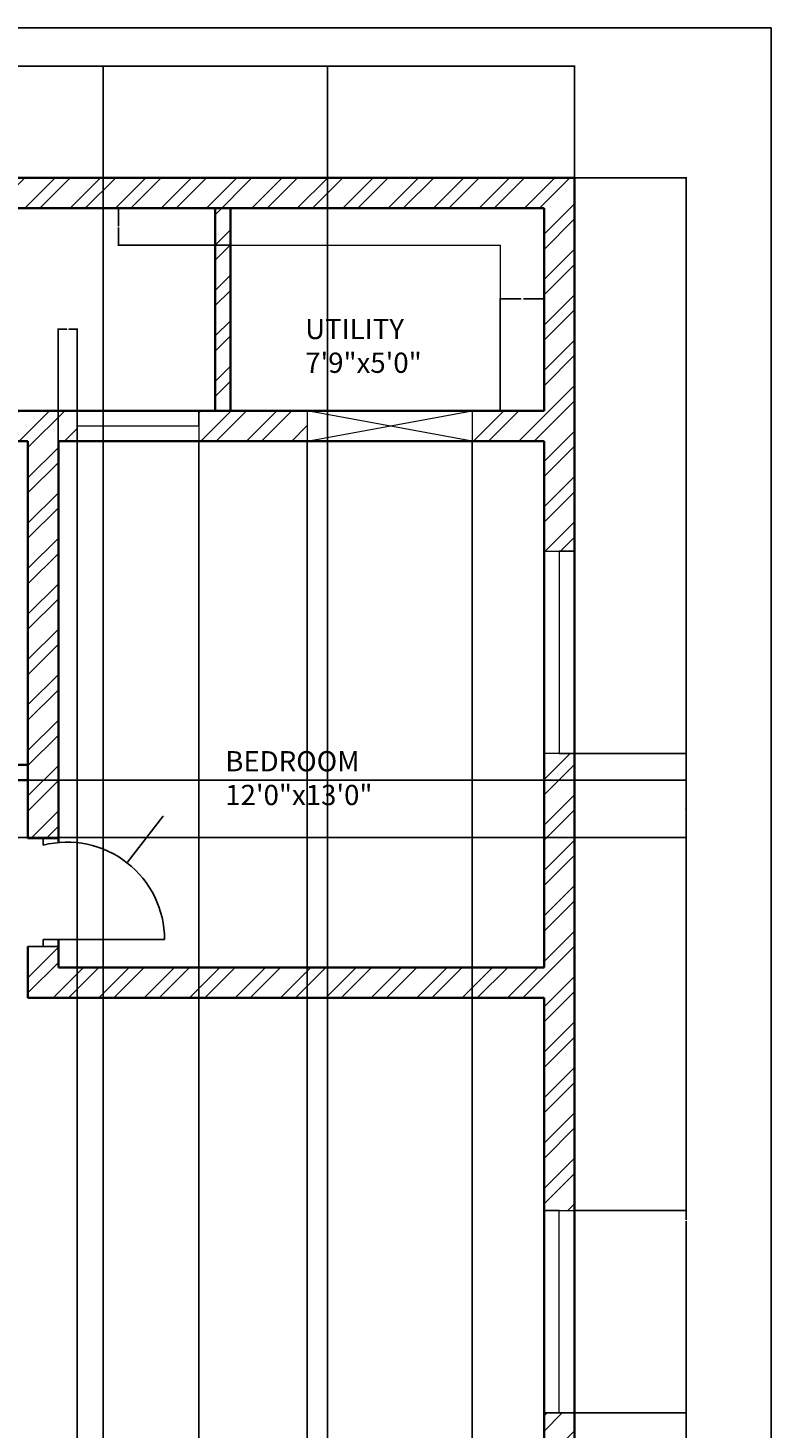
# Model space of a CAD drawing. Units: inches. Extents: x 1595 to 2135, y 460 to 2061.
# Tile 5 of 5: x 1914 to 2135, y 1646 to 2061. Entities that reach past the tile are written whole.
import ezdxf

# ---------------------------------------------------------------- set-up
doc = ezdxf.new("R2010")
doc.units = ezdxf.units.IN
for name, color, linetype, lineweight in [('A-ANNO-DIMS', 2, 'Continuous', 18), ('A-ANNO-TTLB', 7, 'Continuous', 25), ('A-AREA-IDEN', 7, 'Continuous', 18), ('A-DOOR', 3, 'Continuous', 25), ('A-FLOR-FIXT', 9, 'Continuous', 18), ('A-GLAZ', 4, 'Continuous', 18), ('A-WALL', 7, 'Continuous', 35)]:
    doc.layers.add(name, color=color, linetype=linetype, lineweight=lineweight)
doc.layers.add('A-WALL-PATT', color=143, linetype='Continuous', lineweight=13, true_color=0x7aafdf)
doc.styles.get("Standard").update_dxf_attribs({"font": 'arial.ttf'})
doc.dimstyles.get("Standard").update_dxf_attribs({"dimtxt": 0.18, "dimasz": 0.18, "dimexe": 0.18, "dimexo": 0.0625, "dimgap": 0.09, "dimtad": 0, "dimtih": 1, "dimtoh": 1, "dimdec": 4, "dimzin": 0, "dimdsep": 46, "dimtxsty": 'Standard', "dimcen": 0.09, "dimadec": 0, "dimazin": 0, "dimtfac": 1, "dimtdec": 4, "dimtofl": 0, "dimtmove": 0, "dimatfit": 3, "dimfxl": 1, "dimtolj": 1, "dimtzin": 0, "dimarcsym": 0})

# ---------------------------------------------------------------- blocks, each defined once
blk = doc.blocks.new('*D7')
at = {"layer": 'A-ANNO-DIMS', "color": 0, "lineweight": -2, "transparency": 16777216}
for p, q in [((1923.31, 1938.7), (1923.31, 1971.97)), ((1923.49, 1971.79), (1925.8, 1971.79)), ((1928.75, 1971.79), (1926.45, 1971.79)), ((1928.93, 1938.7), (1928.93, 1971.97))]:
    blk.add_line(p, q, dxfattribs=at)
at = {"layer": 'A-ANNO-DIMS', "color": 0, "transparency": 16777216}
for points in [[(1923.49, 1971.82), (1923.49, 1971.76), (1923.31, 1971.79)], [(1928.75, 1971.82), (1928.75, 1971.76), (1928.93, 1971.79)]]:
    blk.add_solid(points, dxfattribs=at)
at = {"layer": 'Defpoints', "color": 0, "transparency": 16777216}
for p in [(1928.93, 1971.79), (1923.31, 1938.64), (1928.93, 1938.64)]:
    blk.add_point(p, dxfattribs=at)
at = {"layer": 'A-ANNO-DIMS', "color": 0, "transparency": 16777216, "insert": (1926.12, 1971.79), "char_height": 0.18, "attachment_point": 5}
blk.add_mtext('\\A1;5.62', dxfattribs=at)
blk = doc.blocks.new('*D15')
at = {"layer": 'A-ANNO-DIMS', "color": 0, "lineweight": -2, "transparency": 16777216}
for p, q in [((2076.38, 1650.64), (2109.64, 1650.64)), ((2109.46, 1650.46), (2109.46, 1577.6)), ((2109.46, 1504.38), (2109.46, 1577.24)), ((2076.38, 1504.2), (2109.64, 1504.2))]:
    blk.add_line(p, q, dxfattribs=at)
at = {"layer": 'A-ANNO-DIMS', "color": 0, "transparency": 16777216}
for points in [[(2109.43, 1650.46), (2109.49, 1650.46), (2109.46, 1650.64)], [(2109.43, 1504.38), (2109.49, 1504.38), (2109.46, 1504.2)]]:
    blk.add_solid(points, dxfattribs=at)
at = {"layer": 'Defpoints', "color": 0, "transparency": 16777216}
for p in [(2076.31, 1650.64), (2109.46, 1650.64), (2076.31, 1504.2)]:
    blk.add_point(p, dxfattribs=at)
at = {"layer": 'A-ANNO-DIMS', "color": 0, "transparency": 16777216, "insert": (2109.46, 1577.42), "char_height": 0.18, "attachment_point": 5}
blk.add_mtext('\\A1;146.44', dxfattribs=at)
blk = doc.blocks.new('*D16')
at = {"layer": 'A-ANNO-DIMS', "color": 0, "lineweight": -2, "transparency": 16777216}
for p, q in [((2076.38, 1846.04), (2109.64, 1846.04)), ((2109.46, 1845.86), (2109.46, 1778.52)), ((2109.46, 1710.82), (2109.46, 1778.16)), ((2076.38, 1710.64), (2109.64, 1710.64))]:
    blk.add_line(p, q, dxfattribs=at)
at = {"layer": 'A-ANNO-DIMS', "color": 0, "transparency": 16777216}
for points in [[(2109.43, 1845.86), (2109.49, 1845.86), (2109.46, 1846.04)], [(2109.43, 1710.82), (2109.49, 1710.82), (2109.46, 1710.64)]]:
    blk.add_solid(points, dxfattribs=at)
at = {"layer": 'Defpoints', "color": 0, "transparency": 16777216}
for p in [(2076.31, 1846.04), (2109.46, 1846.04), (2076.31, 1710.64)]:
    blk.add_point(p, dxfattribs=at)
at = {"layer": 'A-ANNO-DIMS', "color": 0, "transparency": 16777216, "insert": (2109.46, 1778.34), "char_height": 0.18, "attachment_point": 5}
blk.add_mtext('\\A1;135.4', dxfattribs=at)
blk = doc.blocks.new('*D21')
at = {"layer": 'A-ANNO-DIMS', "color": 0, "lineweight": -2, "transparency": 16777216}
for p, q in [((1936.61, 1577.2), (1936.61, 2049.97)), ((1936.79, 2049.79), (1969.47, 2049.79)), ((2002.95, 2049.79), (1970.26, 2049.79)), ((2003.13, 1577.2), (2003.13, 2049.97))]:
    blk.add_line(p, q, dxfattribs=at)
at = {"layer": 'A-ANNO-DIMS', "color": 0, "transparency": 16777216}
for points in [[(1936.79, 2049.82), (1936.79, 2049.76), (1936.61, 2049.79)], [(2002.95, 2049.82), (2002.95, 2049.76), (2003.13, 2049.79)]]:
    blk.add_solid(points, dxfattribs=at)
at = {"layer": 'Defpoints', "color": 0, "transparency": 16777216}
for p in [(2003.13, 2049.79), (1936.61, 1577.14), (2003.13, 1577.14)]:
    blk.add_point(p, dxfattribs=at)
at = {"layer": 'A-ANNO-DIMS', "color": 0, "transparency": 16777216, "insert": (1969.87, 2049.79), "char_height": 0.18, "attachment_point": 5}
blk.add_mtext('\\A1;66.52', dxfattribs=at)
blk = doc.blocks.new('*D27')
at = {"layer": 'A-ANNO-DIMS', "color": 0, "lineweight": -2, "transparency": 16777216}
for p, q in [((1997.11, 1938.58), (1997.11, 1365.31)), ((2046.03, 1938.58), (2046.03, 1365.31)), ((1997.29, 1365.49), (2021.18, 1365.49)), ((2045.85, 1365.49), (2021.97, 1365.49))]:
    blk.add_line(p, q, dxfattribs=at)
at = {"layer": 'A-ANNO-DIMS', "color": 0, "transparency": 16777216}
for points in [[(1997.29, 1365.52), (1997.29, 1365.46), (1997.11, 1365.49)], [(2045.85, 1365.52), (2045.85, 1365.46), (2046.03, 1365.49)]]:
    blk.add_solid(points, dxfattribs=at)
at = {"layer": 'Defpoints', "color": 0, "transparency": 16777216}
for p in [(1997.11, 1938.64), (2046.03, 1938.64), (2046.03, 1365.49)]:
    blk.add_point(p, dxfattribs=at)
at = {"layer": 'A-ANNO-DIMS', "color": 0, "transparency": 16777216, "insert": (2021.57, 1365.49), "char_height": 0.18, "attachment_point": 5}
blk.add_mtext('\\A1;48.92', dxfattribs=at)
blk = doc.blocks.new('*D28')
at = {"layer": 'A-ANNO-DIMS', "color": 0, "lineweight": -2, "transparency": 16777216}
for p, q in [((1928.93, 1938.58), (1928.93, 1365.31)), ((1964.93, 1938.58), (1964.93, 1365.31)), ((1929.11, 1365.49), (1946.71, 1365.49)), ((1964.75, 1365.49), (1947.15, 1365.49))]:
    blk.add_line(p, q, dxfattribs=at)
at = {"layer": 'A-ANNO-DIMS', "color": 0, "transparency": 16777216}
for points in [[(1929.11, 1365.52), (1929.11, 1365.46), (1928.93, 1365.49)], [(1964.75, 1365.52), (1964.75, 1365.46), (1964.93, 1365.49)]]:
    blk.add_solid(points, dxfattribs=at)
at = {"layer": 'Defpoints', "color": 0, "transparency": 16777216}
for p in [(1928.93, 1938.64), (1964.93, 1938.64), (1964.93, 1365.49)]:
    blk.add_point(p, dxfattribs=at)
at = {"layer": 'A-ANNO-DIMS', "color": 0, "transparency": 16777216, "insert": (1946.93, 1365.49), "char_height": 0.18, "attachment_point": 5}
blk.add_mtext('\\A1;36', dxfattribs=at)
blk = doc.blocks.new('*D29')
at = {"layer": 'A-ANNO-DIMS', "color": 0, "lineweight": -2, "transparency": 16777216}
for p, q in [((1964.93, 1938.58), (1964.93, 1365.31)), ((1997.11, 1938.58), (1997.11, 1365.31)), ((1965.11, 1365.49), (1980.63, 1365.49)), ((1996.93, 1365.49), (1981.42, 1365.49))]:
    blk.add_line(p, q, dxfattribs=at)
at = {"layer": 'A-ANNO-DIMS', "color": 0, "transparency": 16777216}
for points in [[(1965.11, 1365.52), (1965.11, 1365.46), (1964.93, 1365.49)], [(1996.93, 1365.52), (1996.93, 1365.46), (1997.11, 1365.49)]]:
    blk.add_solid(points, dxfattribs=at)
at = {"layer": 'Defpoints', "color": 0, "transparency": 16777216}
for p in [(1964.93, 1938.64), (1997.11, 1938.64), (1997.11, 1365.49)]:
    blk.add_point(p, dxfattribs=at)
at = {"layer": 'A-ANNO-DIMS', "color": 0, "transparency": 16777216, "insert": (1981.02, 1365.49), "char_height": 0.18, "attachment_point": 5}
blk.add_mtext('\\A1;32.18', dxfattribs=at)
blk = doc.blocks.new('*D31')
at = {"layer": 'A-ANNO-DIMS', "color": 0, "lineweight": -2, "transparency": 16777216}
for p, q in [((1836.38, 1838.14), (2109.64, 1838.14)), ((2109.46, 1837.96), (2109.46, 1829.81)), ((2109.46, 1821.29), (2109.46, 1829.44)), ((1836.38, 1821.11), (2109.64, 1821.11))]:
    blk.add_line(p, q, dxfattribs=at)
at = {"layer": 'A-ANNO-DIMS', "color": 0, "transparency": 16777216}
for points in [[(2109.43, 1837.96), (2109.49, 1837.96), (2109.46, 1838.14)], [(2109.43, 1821.29), (2109.49, 1821.29), (2109.46, 1821.11)]]:
    blk.add_solid(points, dxfattribs=at)
at = {"layer": 'Defpoints', "color": 0, "transparency": 16777216}
for p in [(1836.31, 1838.14), (1836.31, 1821.11), (2109.46, 1821.11)]:
    blk.add_point(p, dxfattribs=at)
at = {"layer": 'A-ANNO-DIMS', "color": 0, "transparency": 16777216, "insert": (2109.46, 1829.63), "char_height": 0.18, "attachment_point": 5}
blk.add_mtext('\\A1;17.034', dxfattribs=at)
blk = doc.blocks.new('*D45')
at = {"layer": 'A-ANNO-DIMS', "color": 0, "lineweight": -2, "transparency": 16777216}
for p, q in [((1674.31, 2016.7), (1674.31, 2049.97)), ((1674.49, 2049.79), (1875.02, 2049.79)), ((2076.13, 2049.79), (1875.6, 2049.79)), ((2076.31, 2016.7), (2076.31, 2049.97))]:
    blk.add_line(p, q, dxfattribs=at)
at = {"layer": 'A-ANNO-DIMS', "color": 0, "transparency": 16777216}
for points in [[(1674.49, 2049.82), (1674.49, 2049.76), (1674.31, 2049.79)], [(2076.13, 2049.82), (2076.13, 2049.76), (2076.31, 2049.79)]]:
    blk.add_solid(points, dxfattribs=at)
at = {"layer": 'Defpoints', "color": 0, "transparency": 16777216}
for p in [(2076.31, 2049.79), (1674.31, 2016.64), (2076.31, 2016.64)]:
    blk.add_point(p, dxfattribs=at)
at = {"layer": 'A-ANNO-DIMS', "color": 0, "transparency": 16777216, "insert": (1875.31, 2049.79), "char_height": 0.18, "attachment_point": 5}
blk.add_mtext('\\A1;402', dxfattribs=at)
blk = doc.blocks.new('*D46')
at = {"layer": 'A-ANNO-DIMS', "color": 0, "lineweight": -2, "transparency": 16777216}
for p, q in [((2076.38, 2016.64), (2109.64, 2016.64)), ((2109.46, 2016.46), (2109.46, 1707.82)), ((2109.46, 1398.82), (2109.46, 1707.46)), ((2076.38, 1398.64), (2109.64, 1398.64))]:
    blk.add_line(p, q, dxfattribs=at)
at = {"layer": 'A-ANNO-DIMS', "color": 0, "transparency": 16777216}
for points in [[(2109.43, 2016.46), (2109.49, 2016.46), (2109.46, 2016.64)], [(2109.43, 1398.82), (2109.49, 1398.82), (2109.46, 1398.64)]]:
    blk.add_solid(points, dxfattribs=at)
at = {"layer": 'Defpoints', "color": 0, "transparency": 16777216}
for p in [(2076.31, 2016.64), (2109.46, 2016.64), (2076.31, 1398.64)]:
    blk.add_point(p, dxfattribs=at)
at = {"layer": 'A-ANNO-DIMS', "color": 0, "transparency": 16777216, "insert": (2109.46, 1707.64), "char_height": 0.18, "attachment_point": 5}
blk.add_mtext('\\A1;618', dxfattribs=at)
blk = doc.blocks.new('*D51')
at = {"layer": 'A-ANNO-DIMS', "color": 0, "lineweight": -2, "transparency": 16777216}
for p, q in [((2054.32, 1947.7), (2054.32, 1980.97)), ((2054.5, 1980.79), (2060.43, 1980.79)), ((2067.13, 1980.79), (2061.2, 1980.79)), ((2067.31, 1947.7), (2067.31, 1980.97))]:
    blk.add_line(p, q, dxfattribs=at)
at = {"layer": 'A-ANNO-DIMS', "color": 0, "transparency": 16777216}
for points in [[(2054.5, 1980.82), (2054.5, 1980.76), (2054.32, 1980.79)], [(2067.13, 1980.82), (2067.13, 1980.76), (2067.31, 1980.79)]]:
    blk.add_solid(points, dxfattribs=at)
at = {"layer": 'Defpoints', "color": 0, "transparency": 16777216}
for p in [(2067.31, 1980.79), (2054.32, 1947.64), (2067.31, 1947.64)]:
    blk.add_point(p, dxfattribs=at)
at = {"layer": 'A-ANNO-DIMS', "color": 0, "transparency": 16777216, "insert": (2060.82, 1980.79), "char_height": 0.18, "attachment_point": 5}
blk.add_mtext('\\A1;12.99', dxfattribs=at)
blk = doc.blocks.new('*D52')
at = {"layer": 'A-ANNO-DIMS', "color": 0, "lineweight": -2, "transparency": 16777216}
for p, q in [((1974.25, 2007.64), (1940.98, 2007.64)), ((1941.16, 2007.46), (1941.16, 2002.33)), ((1941.16, 1996.84), (1941.16, 2001.97)), ((1974.25, 1996.66), (1940.98, 1996.66))]:
    blk.add_line(p, q, dxfattribs=at)
at = {"layer": 'A-ANNO-DIMS', "color": 0, "transparency": 16777216}
for points in [[(1941.13, 2007.46), (1941.19, 2007.46), (1941.16, 2007.64)], [(1941.13, 1996.84), (1941.19, 1996.84), (1941.16, 1996.66)]]:
    blk.add_solid(points, dxfattribs=at)
at = {"layer": 'Defpoints', "color": 0, "transparency": 16777216}
for p in [(1941.16, 2007.64), (1974.31, 2007.64), (1974.31, 1996.66)]:
    blk.add_point(p, dxfattribs=at)
at = {"layer": 'A-ANNO-DIMS', "color": 0, "transparency": 16777216, "insert": (1941.16, 2002.15), "char_height": 0.18, "attachment_point": 5}
blk.add_mtext('\\A1;10.98', dxfattribs=at)
blk = doc.blocks.new('*D57')
at = {"layer": 'A-ANNO-DIMS', "color": 0, "lineweight": -2, "transparency": 16777216}
for p, q in [((1954.31, 1827.37), (1943.77, 1813.83)), ((1954.49, 1827.37), (1954.31, 1827.37)), ((1925.83, 1790.88), (1926.01, 1790.88)), ((1925.92, 1790.79), (1925.92, 1790.97))]:
    blk.add_line(p, q, dxfattribs=at)
at = {"layer": 'A-ANNO-DIMS', "color": 0, "transparency": 16777216}
blk.add_solid([(1943.75, 1813.85), (1943.8, 1813.81), (1943.66, 1813.69)], dxfattribs=at)
at = {"layer": 'Defpoints', "color": 0, "transparency": 16777216}
for p in [(1943.66, 1813.69), (1925.92, 1790.88)]:
    blk.add_point(p, dxfattribs=at)
at = {"layer": 'A-ANNO-DIMS', "color": 0, "transparency": 16777216, "insert": (1955.04, 1827.37), "char_height": 0.18, "attachment_point": 5}
blk.add_mtext('\\A1;R28.896', dxfattribs=at)

msp = doc.modelspace()

# ---------------------------------------------------------------- hatches: boundary and pattern name
at = {"layer": 'A-WALL-PATT'}
h = msp.add_hatch(dxfattribs=at)
h.set_pattern_fill('ANSI32', color=256)
h.paths.add_polyline_path([(2076.313, 2016.6421), (1674.313, 2016.6421), (1674.313, 1905.0731), (1683.313, 1905.0731), (1683.313, 1938.6421), (1705.9756, 1938.6421), (1705.9756, 1947.6421), (1683.313, 1947.6421), (1683.313, 2007.6421), (2067.313, 2007.6421), (2067.313, 1947.6421), (2046.0304, 1947.6421), (2046.0304, 1938.6421), (2067.313, 1938.6421), (2067.313, 1906.0373), (2076.313, 1906.0373), (2076.313, 1947.6421)])
h.paths.add_polyline_path([(1786.653, 1947.6421), (1748.8699, 1947.6421), (1748.8699, 1938.6421), (1786.653, 1938.6421), (1786.653, 1943.1421)], flags=17)
h.paths.add_polyline_path([(1843.367, 1943.1421), (1843.367, 1947.6421), (1822.653, 1947.6421), (1822.653, 1938.6421), (1827.313, 1938.6421), (1827.313, 1821.1082), (1836.313, 1821.1082), (1836.313, 1938.6421), (1843.367, 1938.6421)])
h.paths.add_polyline_path([(1928.933, 1943.1421), (1928.933, 1947.6421), (1875.313, 1947.6421), (1875.313, 1938.6421), (1914.313, 1938.6421), (1914.313, 1820.8892), (1923.313, 1820.8892), (1923.313, 1938.6421), (1928.933, 1938.6421)])
h.paths.add_polyline_path([(1997.1133, 1947.6421), (1964.933, 1947.6421), (1964.933, 1938.6421), (1997.1133, 1938.6421)], flags=17)
h.paths.add_polyline_path([(1974.313, 2007.6421), (1969.813, 2007.6421), (1969.813, 1947.6421), (1974.313, 1947.6421)], flags=17)
h.paths.add_polyline_path([(1780.813, 2007.6421), (1776.313, 2007.6421), (1776.313, 1947.6421), (1780.813, 1947.6421)], flags=17)
h.paths.add_polyline_path([(1683.313, 1845.0731), (1674.313, 1845.0731), (1674.313, 1734.209), (1683.313, 1734.209), (1683.313, 1773.6421), (1795.813, 1773.6421), (1836.313, 1773.6421), (1836.313, 1788.3627), (1831.813, 1788.3627), (1827.313, 1788.3627), (1827.313, 1782.6421), (1683.313, 1782.6421)])
h.paths.add_polyline_path([(2076.313, 1846.0373), (2067.313, 1846.0373), (2067.313, 1782.6421), (1923.313, 1782.6421), (1923.313, 1788.8802), (1918.813, 1788.8802), (1914.313, 1788.8802), (1914.313, 1773.6421), (2067.313, 1773.6421), (2067.313, 1710.6421), (2076.313, 1710.6421)])
h.paths.add_polyline_path([(1844.0531, 1859.9747), (1909.4596, 1859.9747), (1909.4596, 1882.3635), (1844.0531, 1882.3635)], flags=9)
h.paths.add_polyline_path([(1721.6058, 1827.3507), (1768.2143, 1827.3507), (1768.2143, 1849.7395), (1721.6058, 1849.7395)], flags=9)
h.paths.add_polyline_path([(1786.8661, 1359.2872), (1978.2276, 1359.2872), (1978.2276, 1384.0157), (1786.8661, 1384.0157)], flags=9)
h.paths.add_polyline_path([(1795.7228, 1412.0413), (1871.5904, 1412.0413), (1871.5904, 1424.4055), (1795.7228, 1424.4055)], flags=9)
h.paths.add_polyline_path([(1954.3634, 1526.3976), (2013.549, 1526.3976), (2013.549, 1548.7864), (1954.3634, 1548.7864)], flags=9)
h.paths.add_polyline_path([(1871.0596, 1490.4707), (1913.1292, 1490.4707), (1913.1292, 1512.8595), (1871.0596, 1512.8595)], flags=9)
h.paths.add_polyline_path([(1810.9452, 1510.8402), (1845.9343, 1510.8402), (1845.9343, 1533.229), (1810.9452, 1533.229)], flags=9)
h.paths.add_polyline_path([(1720.9117, 1692.9695), (1767.819, 1692.9695), (1767.819, 1715.3583), (1720.9117, 1715.3583)], flags=9)
h.paths.add_polyline_path([(1853.0254, 1698.4614), (1904.6966, 1698.4614), (1904.6966, 1720.8503), (1853.0254, 1720.8503)], flags=9)
h.paths.add_polyline_path([(1970.399, 1827.3507), (2017.0075, 1827.3507), (2017.0075, 1849.7395), (1970.399, 1849.7395)], flags=9)
h.paths.add_polyline_path([(1994.3418, 1955.5613), (2029.5928, 1955.5613), (2029.5928, 1977.9501), (1994.3418, 1977.9501)], flags=25)
h.paths.add_polyline_path([(1828.8665, 1964.6116), (1868.5173, 1964.6116), (1868.5173, 1987.0004), (1828.8665, 1987.0004)], flags=25)
h.paths.add_polyline_path([(1698.1483, 1960.8371), (1733.3994, 1960.8371), (1733.3994, 1983.2259), (1698.1483, 1983.2259)], flags=25)
h = msp.add_hatch(dxfattribs=at)
h.set_pattern_fill('ANSI32', color=256)
h.paths.add_polyline_path([(1683.313, 1641.6421), (1791.313, 1641.6421), (1791.313, 1634.7169), (1800.313, 1634.7169), (1800.313, 1650.6421), (1800.313, 1673.3054), (1795.813, 1673.3054), (1795.813, 1650.6421), (1683.313, 1650.6421), (1683.313, 1698.209), (1678.813, 1698.209), (1674.313, 1698.209), (1674.313, 1398.6421), (1688.853, 1398.6421), (1688.853, 1403.1421), (1688.853, 1407.6421), (1683.313, 1407.6421)])
h.paths.add_polyline_path([(1800.313, 1568.1421), (1827.2399, 1568.1421), (1827.2399, 1572.6421), (1827.2399, 1577.1421), (1800.313, 1577.1421), (1800.313, 1604.9472), (1795.813, 1604.9472), (1791.313, 1604.9472), (1791.313, 1437.6421), (1800.313, 1437.6421), (1815.6708, 1437.6421), (1815.6708, 1442.1421), (1815.6708, 1446.6421), (1800.313, 1446.6421)])
h.paths.add_polyline_path([(1877.5816, 1545.4284), (1877.5816, 1548.9761), (1864.813, 1548.9761), (1864.813, 1577.1421), (1852.144, 1577.1421), (1852.144, 1568.1421), (1860.313, 1568.1421), (1860.313, 1446.6421), (1839.6708, 1446.6421), (1839.6708, 1437.6421), (1869.0647, 1437.6421), (1869.0647, 1442.1421), (1869.0647, 1446.6421), (1864.813, 1446.6421), (1864.813, 1539.9761), (1877.5816, 1539.9761), (1877.5816, 1541.8808)])
h.paths.add_polyline_path([(1923.313, 1568.1421), (1936.607, 1568.1421), (1936.607, 1577.1421), (1914.313, 1577.1421), (1914.313, 1548.9761), (1901.5816, 1548.9761), (1901.5816, 1539.9761), (1914.313, 1539.9761), (1914.313, 1446.6421), (1891.5684, 1446.6421), (1891.5684, 1437.6421), (1914.313, 1437.6421), (1923.313, 1437.6421)])
h.paths.add_polyline_path([(2067.313, 1577.1421), (2003.1294, 1577.1421), (2003.1294, 1568.1421), (2067.313, 1568.1421)])
h.paths.add_polyline_path([(2076.313, 1650.6421), (2067.313, 1650.6421), (2067.313, 1504.2035), (2076.313, 1504.2035)])
h.paths.add_polyline_path([(2076.313, 1444.2035), (2071.813, 1444.2035), (2067.313, 1444.2035), (2067.313, 1407.6421), (1923.313, 1407.6421), (1918.813, 1407.6421), (1914.313, 1407.6421), (1737.2767, 1407.6421), (1737.2767, 1398.6421), (2076.313, 1398.6421)])

# ---------------------------------------------------------------- linework, layer by layer
at = {"layer": 'A-ANNO-TTLB'}
msp.add_lwpolyline([(1595.2754, 2061.0707), (2134.6206, 2061.0707), (2134.6206, 1319.9937), (1595.2754, 1319.9937)], close=True, dxfattribs=at)
at = {"layer": 'A-DOOR'}
for p, q in [((1914.313, 1820.8892), (1923.313, 1820.8892)), ((1923.313, 1820.8892), (1918.813, 1820.8892)), ((1918.813, 1820.8892), (1918.813, 1818.8892)), ((1914.313, 1788.8802), (1923.313, 1788.8802)), ((1918.813, 1788.8802), (1918.813, 1790.8802)), ((1918.813, 1790.8802), (1954.813, 1790.8802)), ((1918.813, 1790.8802), (1954.813, 1790.8802)), ((1923.313, 1788.8802), (1918.813, 1788.8802))]:
    msp.add_line(p, q, dxfattribs=at)
msp.add_arc((1925.9171, 1790.8802), 28.8959, 360, 104.232183, dxfattribs=at)
at = {"layer": 'A-FLOR-FIXT'}
for p, q in [((1974.313, 1996.6616), (2054.323, 1996.6616)), ((2054.323, 1996.6616), (2054.323, 1947.6421))]:
    msp.add_line(p, q, dxfattribs=at)
at = {"layer": 'A-GLAZ'}
for p, q in [((1928.933, 1947.6421), (1928.933, 1938.6421)), ((1964.933, 1943.1421), (1964.933, 1947.6421)), ((1964.933, 1947.6421), (1964.933, 1938.6421)), ((1997.1133, 1947.6421), (1997.1133, 1938.6421)), ((2046.0304, 1938.6421), (1997.1133, 1947.6421)), ((1997.1133, 1947.6421), (1997.1133, 1947.6421)), ((1997.1133, 1938.6421), (2046.0304, 1947.6421)), ((2046.0304, 1947.6421), (2046.0304, 1938.6421)), ((1928.933, 1938.6421), (1928.933, 1943.1421)), ((1928.933, 1943.1421), (1964.933, 1943.1421)), ((1997.1133, 1938.6421), (1997.1133, 1938.6421)), ((2046.0304, 1938.6421), (2046.0304, 1938.6421)), ((2067.313, 1906.0373), (2076.313, 1906.0373)), ((2076.313, 1906.0373), (2071.813, 1906.0373)), ((2071.813, 1906.0373), (2071.813, 1846.0373)), ((2076.313, 1846.0373), (2067.313, 1846.0373)), ((2071.813, 1846.0373), (2076.313, 1846.0373)), ((2071.813, 1710.6421), (2067.313, 1710.6421)), ((2067.313, 1710.6421), (2076.313, 1710.6421)), ((2071.813, 1650.6421), (2071.813, 1710.6421)), ((2067.313, 1650.6421), (2076.313, 1650.6421)), ((2076.313, 1650.6421), (2067.313, 1650.6421))]:
    msp.add_line(p, q, dxfattribs=at)
at = {"layer": 'A-WALL'}
for p, q in [((1674.313, 2016.6421), (2076.313, 2016.6421)), ((2076.313, 2016.6421), (2076.313, 1947.6421)), ((1683.313, 2007.6421), (2067.313, 2007.6421)), ((1969.813, 2007.6421), (1969.813, 1947.6421)), ((1974.313, 2007.6421), (1974.313, 1947.6421)), ((2067.313, 2007.6421), (2067.313, 1947.6421)), ((1875.313, 1947.6421), (2067.313, 1947.6421)), ((2076.313, 1947.6421), (2076.313, 1398.6421)), ((1874.0917, 1938.6421), (1914.313, 1938.6421)), ((1914.313, 1938.6421), (1914.313, 1820.8892)), ((1923.313, 1938.6421), (1923.313, 1819.6585)), ((1923.313, 1938.6421), (2067.313, 1938.6421)), ((2067.313, 1782.6421), (2067.313, 1938.6421)), ((1836.313, 1842.6421), (1914.313, 1842.6421)), ((1836.313, 1838.1421), (1914.313, 1838.1421)), ((1914.313, 1788.8802), (1914.313, 1773.6421)), ((1923.313, 1790.8802), (1923.313, 1782.6421)), ((1923.313, 1782.6421), (2067.313, 1782.6421)), ((1914.313, 1773.6421), (2067.313, 1773.6421)), ((2067.313, 1650.6421), (2067.313, 1773.6421)), ((2067.313, 1407.6421), (2067.313, 1650.6421))]:
    msp.add_line(p, q, dxfattribs=at)

# ---------------------------------------------------------------- texts
at = {"layer": 'A-AREA-IDEN', "char_height": 6, "attachment_point": 1}
for s, width, insert in [('UTILITY\\P7\'9"x5\'0"', 175.461438, (1996.5007, 1974.8621)), ('BEDROOM\\P12\'0"x13\'0"', 157.676153, (1972.8117, 1846.7579))]:
    msp.add_mtext_dynamic_manual_height_columns(s, width=width, gutter_width=12.5, heights=[0], dxfattribs=dict(at, insert=insert))

# ---------------------------------------------------------------- dimensions: what is measured, and where the dimension line sits
at = {"layer": 'A-ANNO-DIMS'}
for base, p1, p2, override, picture, middle in [((2076.313, 2049.7921), (1674.313, 2016.6421), (2076.313, 2016.6421), {"dimdec": 0, "dimlfac": 1, "dimrnd": 0, "dimzin": 0, "dimdsep": 46, "dimlunit": 2}, '*D45', (1875.313, 2049.7921)), ((2003.1294, 2049.7921), (1936.607, 1577.1421), (2003.1294, 1577.1421), {"dimdec": 2, "dimlfac": 1, "dimrnd": 0, "dimzin": 0, "dimdsep": 46, "dimlunit": 2}, '*D21', (1969.8682, 2049.7921)), ((2067.313, 1980.7921), (2054.323, 1947.6421), (2067.313, 1947.6421), {"dimdec": 2, "dimlfac": 1, "dimrnd": 0, "dimzin": 0, "dimdsep": 46, "dimlunit": 2}, '*D51', (2060.818, 1980.7921)), ((1928.933, 1971.7921), (1923.313, 1938.6421), (1928.933, 1938.6421), {"dimdec": 2, "dimlfac": 1, "dimrnd": 0, "dimzin": 0, "dimdsep": 46, "dimlunit": 2}, '*D7', (1926.123, 1971.7921)), ((1964.933, 1365.4921), (1928.933, 1938.6421), (1964.933, 1938.6421), {"dimdec": 0, "dimlfac": 1, "dimrnd": 0, "dimzin": 0, "dimdsep": 46, "dimlunit": 2}, '*D28', (1946.933, 1365.4921)), ((1997.1133, 1365.4921), (1964.933, 1938.6421), (1997.1133, 1938.6421), {"dimdec": 2, "dimlfac": 1, "dimrnd": 0, "dimzin": 0, "dimdsep": 46, "dimlunit": 2}, '*D29', (1981.0231, 1365.4921)), ((2046.0304, 1365.4921), (1997.1133, 1938.6421), (2046.0304, 1938.6421), {"dimdec": 2, "dimlfac": 1, "dimrnd": 0, "dimzin": 0, "dimdsep": 46, "dimlunit": 2}, '*D27', (2021.5719, 1365.4921))]:
    dim = msp.add_linear_dim(base=base, p1=p1, p2=p2, dimstyle='Standard', override=override, dxfattribs=at)
    dim.commit()
    dim.dimension.update_dxf_attribs({"geometry": picture, "text_midpoint": middle})
for base, p1, p2, override, picture, middle in [((2109.463, 2016.6421), (2076.313, 1398.6421), (2076.313, 2016.6421), {"dimdec": 0, "dimlfac": 1, "dimrnd": 0, "dimzin": 0, "dimdsep": 46, "dimlunit": 2}, '*D46', (2109.463, 1707.6421)), ((1941.163, 2007.6421), (1974.313, 1996.6616), (1974.313, 2007.6421), {"dimdec": 2, "dimlfac": 1, "dimrnd": 0, "dimzin": 0, "dimdsep": 46, "dimlunit": 2}, '*D52', (1941.163, 2002.1518)), ((2109.463, 1846.0373), (2076.313, 1710.6421), (2076.313, 1846.0373), {"dimdec": 1, "dimlfac": 1, "dimrnd": 0, "dimzin": 0, "dimdsep": 46, "dimlunit": 2}, '*D16', (2109.463, 1778.3397)), ((2109.463, 1821.1082), (1836.313, 1838.1421), (1836.313, 1821.1082), {"dimdec": 3, "dimlfac": 1, "dimrnd": 0, "dimzin": 0, "dimdsep": 46, "dimlunit": 2}, '*D31', (2109.463, 1829.6251)), ((2109.463, 1650.6421), (2076.313, 1504.2035), (2076.313, 1650.6421), {"dimdec": 2, "dimlfac": 1, "dimrnd": 0, "dimzin": 0, "dimdsep": 46, "dimlunit": 2}, '*D15', (2109.463, 1577.4228))]:
    dim = msp.add_linear_dim(base=base, p1=p1, p2=p2, angle=90, dimstyle='Standard', override=override, dxfattribs=at)
    dim.commit()
    dim.dimension.update_dxf_attribs({"geometry": picture, "text_midpoint": middle})
dim = msp.add_radius_dim(center=(1925.9171, 1790.8802), mpoint=(1943.6613, 1813.6863), dimstyle='Standard', override={"dimdec": 3, "dimlfac": 1, "dimrnd": 0, "dimzin": 0, "dimdsep": 46, "dimlunit": 2}, dxfattribs=at)
dim.commit()
dim.dimension.update_dxf_attribs({"geometry": '*D57', "text_midpoint": (1955.0374, 1827.37), "dimtype": 164})

doc.saveas('drawing.dxf')
